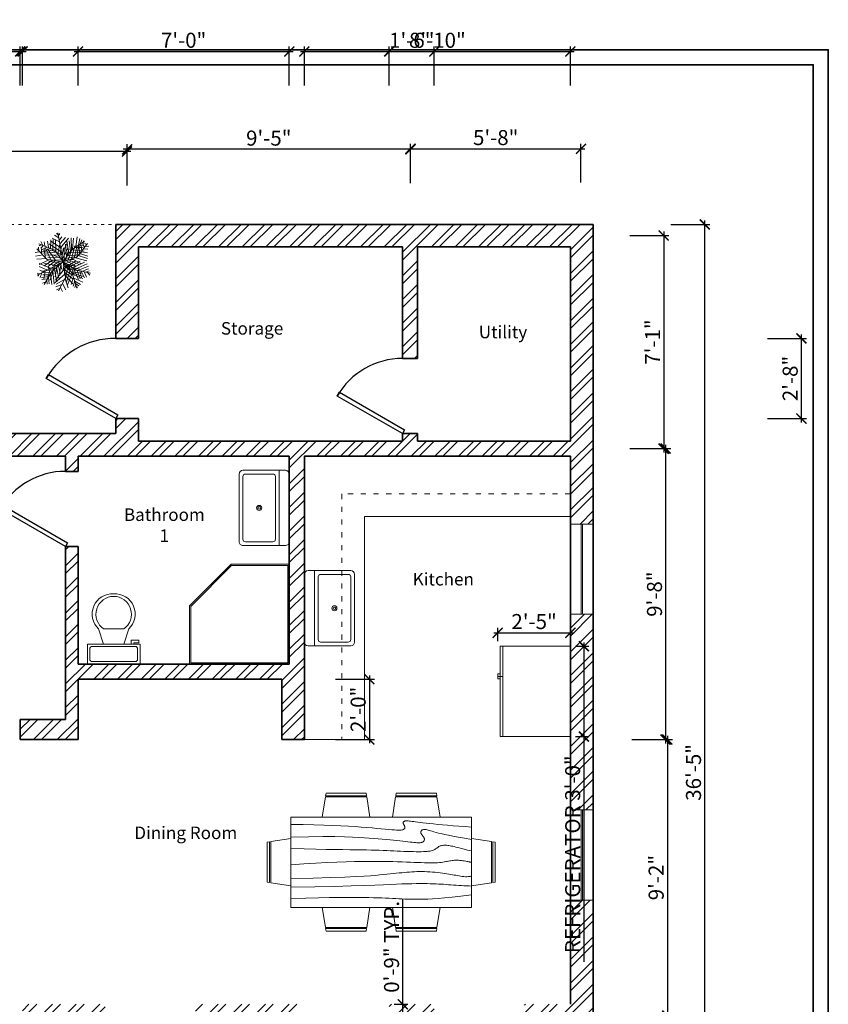
# Model space of a CAD drawing. Units: inches. Extents: x 163 to 947, y 159 to 804.
# Tile 5 of 5: x 625 to 947, y 412 to 804. Entities that reach past the tile are written whole.
import ezdxf

# ---------------------------------------------------------------- set-up
doc = ezdxf.new("R2010")
doc.units = ezdxf.units.IN
doc.linetypes.add('ACAD_ISO03W100', pattern=[30, 12, -18])
for name, color, linetype, lineweight in [('A-ANNO-TTLB', 7, 'Continuous', 35), ('A-AREA-IDEN', 7, 'Continuous', 18), ('A-EQPM', 121, 'Continuous', 18), ('A-FLOR-CASE', 7, 'Continuous', 18), ('A-FLOR-CASE-OVHD', 7, 'ACAD_ISO03W100', 18), ('A-FLOR-FIXT', 121, 'Continuous', 18), ('A-ROOF-OVHD', 7, 'ACAD_ISO03W100', 18), ('Dimensions', 7, 'Continuous', 18), ('Doors', 160, 'Continuous', 25), ('Furniture', 40, 'Continuous', 18), ('Greenary  Plants', 100, 'Continuous', 13), ('Wall Hatch', 214, 'Continuous', 13), ('Walls', 222, 'Continuous', 35), ('Windows', 132, 'Continuous', 18)]:
    doc.layers.add(name, color=color, linetype=linetype, lineweight=lineweight)
doc.styles.get("Standard").update_dxf_attribs({"font": 'arial.ttf'})
doc.dimstyles.new('ISO-25', dxfattribs={"dimtxt": 6, "dimasz": 4, "dimexe": 2, "dimexo": 2, "dimtad": 1, "dimdec": 1, "dimlunit": 3, "dimtxsty": 'Standard', "dimblk": 'ARCHTICK', "dimcen": 0, "dimdle": 1.5, "dimadec": 0, "dimazin": 0, "dimtfac": 1, "dimtdec": 1, "dimtmove": 0, "dimatfit": 3, "dimfxl": 13.5, "dimfxlon": 1, "dimarcsym": 0})

# ---------------------------------------------------------------- blocks, each defined once
blk = doc.blocks.new('_ArchTick')
at = {"color": 0, "linetype": 'ByBlock', "const_width": 0.15}
blk.add_lwpolyline([(-0.5, -0.5), (0.5, 0.5)], dxfattribs=at)
blk = doc.blocks.new('*D2')
at = {"layer": 'Dimensions', "color": 0, "lineweight": -2, "transparency": 16777216}
for p, q in [((780.8, 739.36), (780.8, 754.86)), ((848.8, 739.36), (848.8, 754.86)), ((779.3, 752.86), (850.3, 752.86))]:
    blk.add_line(p, q, dxfattribs=at)
at = {"layer": 'Dimensions', "color": 0, "lineweight": -2, "transparency": 16777216, "xscale": 4, "yscale": 4, "zscale": 4, "rotation": 180}
blk.add_blockref('_ArchTick', (780.8, 752.86), dxfattribs=at)
at = {"layer": 'Dimensions', "color": 0, "lineweight": -2, "transparency": 16777216, "xscale": 4, "yscale": 4, "zscale": 4}
blk.add_blockref('_ArchTick', (848.8, 752.86), dxfattribs=at)
at = {"layer": 'Dimensions', "color": 0, "transparency": 16777216, "insert": (814.8, 756.55), "char_height": 6, "attachment_point": 5}
blk.add_mtext('5\'-8"', dxfattribs=at)
blk = doc.blocks.new('*D3')
at = {"layer": 'Dimensions', "color": 0, "lineweight": -2, "transparency": 16777216}
for p, q in [((667.8, 739.15), (667.8, 754.65)), ((780.8, 739.15), (780.8, 754.65)), ((782.3, 752.65), (666.3, 752.65))]:
    blk.add_line(p, q, dxfattribs=at)
at = {"layer": 'Dimensions', "color": 0, "lineweight": -2, "transparency": 16777216, "xscale": 4, "yscale": 4, "zscale": 4, "rotation": 180}
blk.add_blockref('_ArchTick', (667.8, 752.65), dxfattribs=at)
at = {"layer": 'Dimensions', "color": 0, "lineweight": -2, "transparency": 16777216, "xscale": 4, "yscale": 4, "zscale": 4}
blk.add_blockref('_ArchTick', (780.8, 752.65), dxfattribs=at)
at = {"layer": 'Dimensions', "color": 0, "transparency": 16777216, "insert": (724.3, 756.34), "char_height": 6, "attachment_point": 5}
blk.add_mtext('9\'-5"', dxfattribs=at)
blk = doc.blocks.new('*D4')
at = {"layer": 'Dimensions', "color": 0, "lineweight": -2, "transparency": 16777216}
for p, q in [((542.8, 738.28), (542.8, 753.78)), ((667.8, 738.28), (667.8, 753.78)), ((669.3, 751.78), (541.3, 751.78))]:
    blk.add_line(p, q, dxfattribs=at)
at = {"layer": 'Dimensions', "color": 0, "lineweight": -2, "transparency": 16777216, "xscale": 4, "yscale": 4, "zscale": 4, "rotation": 180}
blk.add_blockref('_ArchTick', (542.8, 751.78), dxfattribs=at)
at = {"layer": 'Dimensions', "color": 0, "lineweight": -2, "transparency": 16777216, "xscale": 4, "yscale": 4, "zscale": 4}
blk.add_blockref('_ArchTick', (667.8, 751.78), dxfattribs=at)
at = {"layer": 'Dimensions', "color": 0, "transparency": 16777216, "insert": (605.3, 755.47), "char_height": 6, "attachment_point": 5}
blk.add_mtext('10\'-5"', dxfattribs=at)
blk = doc.blocks.new('*D8')
at = {"layer": 'Dimensions', "color": 0, "lineweight": -2, "transparency": 16777216}
for p, q in [((881.79, 719.82), (881.79, 631.82)), ((868.29, 718.32), (883.79, 718.32)), ((868.29, 633.32), (883.79, 633.32))]:
    blk.add_line(p, q, dxfattribs=at)
at = {"layer": 'Dimensions', "color": 0, "lineweight": -2, "transparency": 16777216, "xscale": 4, "yscale": 4, "zscale": 4}
for p, rotation in [((881.79, 718.32), 90), ((881.79, 633.32), 270)]:
    blk.add_blockref('_ArchTick', p, dxfattribs=dict(at, rotation=rotation))
at = {"layer": 'Dimensions', "color": 0, "transparency": 16777216, "insert": (878.15, 675.82), "char_height": 6, "attachment_point": 5, "rotation": 90}
blk.add_mtext('7\'-1"', dxfattribs=at)
blk = doc.blocks.new('*D9')
at = {"layer": 'Dimensions', "color": 0, "lineweight": -2, "transparency": 16777216}
for p, q in [((869.08, 633.32), (884.58, 633.32)), ((882.58, 634.82), (882.58, 515.82)), ((869.08, 517.32), (884.58, 517.32))]:
    blk.add_line(p, q, dxfattribs=at)
at = {"layer": 'Dimensions', "color": 0, "lineweight": -2, "transparency": 16777216, "xscale": 4, "yscale": 4, "zscale": 4}
for p, rotation in [((882.58, 633.32), 90), ((882.58, 517.32), 270)]:
    blk.add_blockref('_ArchTick', p, dxfattribs=dict(at, rotation=rotation))
at = {"layer": 'Dimensions', "color": 0, "transparency": 16777216, "insert": (878.9, 575.32), "char_height": 6, "attachment_point": 5, "rotation": 90}
blk.add_mtext('9\'-8"', dxfattribs=at)
blk = doc.blocks.new('*D10')
at = {"layer": 'Dimensions', "color": 0, "lineweight": -2, "transparency": 16777216}
for p, q in [((883.25, 518.82), (883.25, 405.78)), ((869.75, 517.32), (885.25, 517.32)), ((869.75, 407.28), (885.25, 407.28))]:
    blk.add_line(p, q, dxfattribs=at)
at = {"layer": 'Dimensions', "color": 0, "lineweight": -2, "transparency": 16777216, "xscale": 4, "yscale": 4, "zscale": 4}
for p, rotation in [((883.25, 517.32), 90), ((883.25, 407.28), 270)]:
    blk.add_blockref('_ArchTick', p, dxfattribs=dict(at, rotation=rotation))
at = {"layer": 'Dimensions', "color": 0, "transparency": 16777216, "insert": (879.57, 462.3), "char_height": 6, "attachment_point": 5, "rotation": 90}
blk.add_mtext('9\'-2"', dxfattribs=at)
blk = doc.blocks.new('*U25')
for p, q in [((-30, 0), (-30, 4)), ((0, 0), (0, 4))]:
    blk.add_line(p, q)
blk.add_lwpolyline([(0, 0), (-15, -25.98), (-16.52, -25.11), (-1.52, 0.87)], close=True)
blk.add_arc((0, 0), 30, 180, 240)
blk = doc.blocks.new('*U26')
for p, q in [((-32, 0), (-32, 4)), ((0, 0), (0, 4))]:
    blk.add_line(p, q)
blk.add_lwpolyline([(0, 0), (-16, -27.71), (-17.52, -26.84), (-1.52, 0.87)], close=True)
blk.add_arc((0, 0), 32, 180, 240)
blk = doc.blocks.new('Dining Set - 36 x 72 in.')
for p, q in [((-22, 27.5), (-22.1562, 26.50042)), ((-22, 27.5), (-6, 27.5)), ((-5.8437, 26.49966), (-6, 27.5)), ((6, 27.5), (5.8438, 26.50042)), ((6, 27.5), (22, 27.5)), ((22.1563, 26.49966), (22, 27.5)), ((-22.2343, 26.00059), (-23.4847, 17.99762)), ((-22.2304, 26), (-5.7608, 26)), ((-5.8416, 26.5), (-22.1534, 26.5)), ((-4.5152, 17.99762), (-5.7655, 25.99926)), ((5.7657, 26.00059), (4.5153, 17.99762)), ((5.7696, 26), (22.2392, 26)), ((22.1584, 26.5), (5.8466, 26.5)), ((23.4848, 17.99762), (22.2345, 25.99926)), ((36, 18), (-36, 18)), ((-36, 18), (-36, -18)), ((36, -18), (36, 18)), ((-45.5, 8), (-44.5004, 8.15617)), ((-45.5, 8), (-45.5, -8)), ((-44.5, -8.15843), (-44.5, 8.15338)), ((-44.0006, 8.23428), (-35.9976, 9.48474)), ((-44, 8.23041), (-44, -8.23915)), ((44.0006, 8.23428), (35.9976, 9.48474)), ((44, 8.23041), (44, -8.23915)), ((44.5, -8.15843), (44.5, 8.15338)), ((45.5, 8), (44.5005, 8.15617)), ((45.5, 8), (45.5, -8)), ((-44.4997, -8.15631), (-45.5, -8)), ((-35.9976, -9.48476), (-43.9993, -8.2345)), ((35.9976, -9.48476), (43.9993, -8.2345)), ((44.4997, -8.15631), (45.5, -8)), ((-36, -18), (36, -18)), ((-22.2343, -26.0006), (-23.4847, -17.99762)), ((-4.5152, -17.99762), (-5.7655, -25.99928)), ((5.7657, -26.0006), (4.5153, -17.99762)), ((23.4848, -17.99762), (22.2345, -25.99928)), ((-22.2304, -26), (-5.7608, -26)), ((-22, -27.5), (-22.1562, -26.50044)), ((-5.8416, -26.5), (-22.1534, -26.5)), ((-5.8437, -26.49967), (-6, -27.5)), ((5.7696, -26), (22.2392, -26)), ((6, -27.5), (5.8438, -26.50044)), ((22.1584, -26.5), (5.8466, -26.5)), ((22.1563, -26.49967), (22, -27.5)), ((-22, -27.5), (-6, -27.5)), ((6, -27.5), (22, -27.5))]:
    blk.add_line(p, q)
for points in [[(-36, 15), (-31.1772, 14.97754), (-26.8079, 14.91406), (-22.8538, 14.81543), (-19.276, 14.6875), (-16.0362, 14.53613), (-13.0957, 14.36718), (-10.4159, 14.18652), (-7.9583, 14), (-5.6904, 13.81315), (-3.6035, 13.63021), (-1.6954, 13.45508), (0.0365, 13.29166), (1.5945, 13.14388), (2.9811, 13.01562), (4.1988, 12.9108), (5.25, 12.83333), (6.1393, 12.78613), (6.8802, 12.76823), (7.4883, 12.77767), (7.9792, 12.8125), (8.3685, 12.87077), (8.6719, 12.95052), (8.9049, 13.0498), (9.0833, 13.16666), (9.2205, 13.29899), (9.3216, 13.44401), (9.3895, 13.59879), (9.4271, 13.76041), (9.4373, 13.92594), (9.4232, 14.09245), (9.3875, 14.257), (9.3333, 14.41666), (9.2638, 14.56917), (9.1836, 14.71484), (9.0975, 14.85465), (9.0104, 14.98958), (8.9272, 15.1206), (8.8529, 15.2487), (8.7922, 15.37483), (8.75, 15.5), (8.7305, 15.62467), (8.7344, 15.74739), (8.7617, 15.86621), (8.8125, 15.97916), (8.8867, 16.08431), (8.9844, 16.17968), (9.1055, 16.26334), (9.25, 16.33333), (9.4189, 16.38802), (9.6172, 16.42708), (9.8506, 16.45052), (10.125, 16.45833), (10.4463, 16.45052), (10.8203, 16.42708), (11.2529, 16.38802), (11.75, 16.33333), (12.3184, 16.26318), (12.9694, 16.17838), (13.7151, 16.07991), (14.5677, 15.96875), (15.5395, 15.84586), (16.6426, 15.71224), (17.8893, 15.56884), (19.2917, 15.41666), (20.859, 15.25667), (22.5879, 15.08984), (24.4721, 14.91715), (26.5052, 14.73958), (28.6809, 14.5581), (30.9929, 14.3737), (33.4347, 14.18733), (36, 14)], [(-36, 10), (-28.9766, 10.14274), (-23.1725, 10.20442), (-18.4241, 10.19775), (-14.5677, 10.13541), (-11.4399, 10.03011), (-8.877, 9.89453), (-6.7154, 9.74137), (-4.7917, 9.58333), (-2.9698, 9.43082), (-1.2246, 9.28515), (0.4415, 9.14534), (2.026, 9.01041), (3.5266, 8.87939), (4.9408, 8.7513), (6.266, 8.62516), (7.5, 8.5), (8.6411, 8.37549), (9.6914, 8.2539), (10.6538, 8.13818), (11.5312, 8.03125), (12.3267, 7.93603), (13.043, 7.85547), (13.6831, 7.79248), (14.25, 7.75), (14.7471, 7.7303), (15.1797, 7.73307), (15.5537, 7.75732), (15.875, 7.80208), (16.1494, 7.86637), (16.3828, 7.94922), (16.5811, 8.04964), (16.75, 8.16666), (16.8944, 8.29915), (17.0143, 8.44531), (17.1089, 8.60319), (17.1771, 8.77083), (17.218, 8.94629), (17.2305, 9.1276), (17.2137, 9.31282), (17.1667, 9.5), (17.0895, 9.6875), (16.987, 9.875), (16.8649, 10.0625), (16.7292, 10.25), (16.5856, 10.4375), (16.4401, 10.625), (16.2985, 10.8125), (16.1667, 11), (16.05, 11.18733), (15.9518, 11.3737), (15.8752, 11.5581), (15.8229, 11.73958), (15.798, 11.91715), (15.8034, 12.08984), (15.842, 12.25667), (15.9167, 12.41666), (16.0295, 12.56836), (16.1784, 12.70833), (16.3605, 12.83268), (16.5729, 12.9375), (16.8127, 13.01888), (17.0768, 13.07291), (17.3625, 13.0957), (17.6667, 13.08333), (17.9894, 13.03312), (18.3418, 12.94726), (18.7382, 12.82918), (19.1927, 12.68229), (19.7195, 12.51001), (20.3327, 12.31575), (21.0465, 12.10294), (21.875, 11.875), (22.8357, 11.63354), (23.959, 11.37304), (25.2786, 11.08618), (26.8282, 10.76562), (28.6414, 10.40405), (30.752, 9.99414), (33.1936, 9.52856), (36, 9)], [(-36, 5.5), (-30.7157, 5.3348), (-26.069, 5.20963), (-21.9946, 5.11767), (-18.4271, 5.05208), (-15.3009, 5.00602), (-12.5508, 4.97265), (-10.1112, 4.94515), (-7.9167, 4.91666), (-5.909, 4.88167), (-4.0586, 4.83984), (-2.3429, 4.79215), (-0.7396, 4.73958), (0.7739, 4.6831), (2.22, 4.6237), (3.6213, 4.56233), (5, 4.5), (6.373, 4.43782), (7.7344, 4.3776), (9.0723, 4.32129), (10.375, 4.27083), (11.6309, 4.22819), (12.8281, 4.19531), (13.9551, 4.17415), (15, 4.16666), (15.954, 4.17448), (16.819, 4.19791), (17.6001, 4.23698), (18.3021, 4.29166), (18.9299, 4.36198), (19.4883, 4.44791), (19.9823, 4.54948), (20.4167, 4.66666), (20.7969, 4.79899), (21.1302, 4.94401), (21.4245, 5.09879), (21.6875, 5.26041), (21.9271, 5.42594), (22.1511, 5.59245), (22.3672, 5.757), (22.5834, 5.91666), (22.8065, 6.06868), (23.0404, 6.21093), (23.2879, 6.34147), (23.5521, 6.45833), (23.8358, 6.55957), (24.142, 6.64323), (24.4735, 6.70735), (24.8334, 6.75), (25.2235, 6.76969), (25.642, 6.76692), (26.0858, 6.74267), (26.5521, 6.69791), (27.0379, 6.63362), (27.5404, 6.55078), (28.0565, 6.45036), (28.5834, 6.33333), (29.1242, 6.19987), (29.7071, 6.04687), (30.3661, 5.87044), (31.1354, 5.66666), (32.0493, 5.43164), (33.142, 5.16146), (34.4475, 4.85221), (36, 4.5)], [(-36, -1), (-30.7915, -0.6591), (-26.0195, -0.38216), (-21.6519, -0.16284), (-17.6563, 0.00521), (-14.0005, 0.12833), (-10.6523, 0.21289), (-7.5796, 0.26522), (-4.75, 0.29166), (-2.134, 0.29793), (0.2878, 0.28711), (2.5317, 0.26163), (4.6146, 0.22396), (6.5529, 0.17651), (8.3633, 0.12174), (10.0623, 0.06209), (11.6667, 0), (13.1899, -0.06201), (14.6341, -0.1211), (15.9982, -0.17432), (17.2813, -0.21875), (18.4823, -0.25147), (19.6003, -0.26953), (20.6343, -0.27002), (21.5834, -0.25), (22.4481, -0.20768), (23.2357, -0.14584), (23.9549, -0.06836), (24.6146, 0.02083), (25.2235, 0.11784), (25.7904, 0.21875), (26.3241, 0.31966), (26.8334, 0.41666), (27.3265, 0.50618), (27.8099, 0.58593), (28.2894, 0.65397), (28.7709, 0.70833), (29.2601, 0.74707), (29.763, 0.76823), (30.2855, 0.76985), (30.8334, 0.75), (31.4088, 0.70784), (31.9994, 0.64713), (32.589, 0.57275), (33.1615, 0.48958), (33.7008, 0.4025), (34.1908, 0.3164), (34.6153, 0.23616), (34.9584, 0.16666), (35.2099, 0.11165), (35.3848, 0.07031), (35.504, 0.04069), (35.5886, 0.02083), (35.6594, 0.00879), (35.7377, 0.0026), (35.8442, 0.00032), (36, 0)], [(-36, -6.5), (-27.1843, -6.31267), (-20.084, -6.1263), (-14.469, -5.9419), (-10.1094, -5.76042), (-6.7752, -5.58285), (-4.2363, -5.41016), (-2.2629, -5.24333), (-0.625, -5.08334), (0.8708, -4.93099), (2.2715, -4.78646), (3.5872, -4.64974), (4.8281, -4.52084), (6.0046, -4.39974), (7.127, -4.28646), (8.2053, -4.18099), (9.25, -4.08334), (10.2705, -3.99382), (11.2734, -3.91407), (12.2647, -3.84603), (13.25, -3.79167), (14.2354, -3.75293), (15.2266, -3.73177), (16.2295, -3.73015), (17.25, -3.75), (18.2912, -3.79248), (19.3451, -3.85547), (20.4009, -3.93604), (21.4479, -4.03125), (22.4754, -4.13819), (23.4727, -4.25391), (24.4289, -4.37549), (25.3334, -4.5), (26.1785, -4.62492), (26.9694, -4.74935), (27.7145, -4.87281), (28.4219, -4.99479), (29.1, -5.11483), (29.7572, -5.23242), (30.4016, -5.34709), (31.0417, -5.45834), (31.6837, -5.56437), (32.3262, -5.65821), (32.9658, -5.73153), (33.599, -5.77604), (34.2224, -5.78345), (34.8327, -5.74545), (35.4264, -5.65373), (36, -5.5)], [(-36, -10), (-26.4022, -9.81299), (-18.4675, -9.62891), (-11.9839, -9.45069), (-6.7396, -9.28125), (-2.5226, -9.12354), (0.8789, -8.98047), (3.6769, -8.85498), (6.0833, -8.75), (8.2767, -8.66765), (10.3021, -8.60677), (12.1712, -8.56543), (13.8958, -8.54167), (15.4876, -8.53353), (16.9583, -8.53907), (18.3197, -8.55632), (19.5834, -8.58334), (20.7616, -8.61841), (21.8685, -8.66081), (22.9188, -8.71004), (23.9271, -8.76563), (24.9081, -8.82707), (25.8763, -8.89388), (26.8465, -8.96558), (27.8334, -9.04167), (28.8474, -9.12118), (29.8828, -9.20117), (30.93, -9.27824), (31.9792, -9.34896), (33.0205, -9.40991), (34.0443, -9.45768), (35.0407, -9.48885), (36, -9.5)], [(-36, -14.5), (-30.0881, -14.33513), (-25.0332, -14.21224), (-20.7312, -14.12647), (-17.0781, -14.07292), (-13.97, -14.04671), (-11.3027, -14.04297), (-8.9724, -14.05681), (-6.875, -14.08334), (-4.9224, -14.11833), (-3.0905, -14.16016), (-1.3709, -14.20785), (0.2448, -14.26042), (1.7647, -14.3169), (3.1973, -14.3763), (4.5507, -14.43767), (5.8333, -14.5), (7.0554, -14.5621), (8.235, -14.62175), (9.3922, -14.67652), (10.5469, -14.72396), (11.7192, -14.76164), (12.929, -14.78711), (14.1965, -14.79794), (15.5417, -14.79167), (16.9933, -14.76424), (18.6152, -14.70508), (20.4804, -14.60197), (22.6615, -14.44271), (25.2312, -14.21509), (28.2624, -13.9069), (31.8277, -13.50594), (36, -13)]]:
    blk.add_lwpolyline(points)
blk = doc.blocks.new('*U50')
for p, q in [((9.5, -6), (9.5, -2)), ((-10, -8.5), (-8, -8.5)), ((-10, -9.5), (-10, -8.5)), ((-7, -9.5), (-10, -9.5)), ((-8, -8.5), (-8, -8)), ((-7, -8), (-7, -9.5)), ((-4, -8), (-6, -14)), ((4, -8), (6, -14)), ((4, -14), (-4, -14))]:
    blk.add_line(p, q)
blk.add_lwpolyline([(10.5, -8), (10.5, 0), (-10.5, 0), (-10.5, -8)], close=True)
for points in [[(-9.5, -2), (-9.5, -6)], [(8.5, -1), (-8.5, -1)], [(-8.5, -7), (8.5, -7)]]:
    blk.add_lwpolyline(points)
for centre, radius, start, end in [((-8.625, -1.875), 0.8839, 81.8699, 188.1301), ((8.625, -1.875), 0.8839, 351.8699, 98.1301), ((-8.625, -6.125), 0.8839, 171.869898, 278.1301), ((8.625, -6.125), 0.8839, 261.8699, 8.1301), ((-0.4772, -19.9188), 8.0953, 133.01722, 273.38), ((0.0374, -19.8731), 7.127, 124.50543, 269.7), ((-0.0373, -19.8731), 7.127, 270.3, 55.4946), ((0.4773, -19.9188), 8.0953, 266.62, 46.9828)]:
    blk.add_arc(centre, radius, start, end)
blk = doc.blocks.new('Sink-single - 30 in top')
blk.add_line((-15, -3.999996), (15, -3.999996))
for points in [[(-13.5, 0), (13.5, 0)], [(-15, -18.499996), (-15, -1.5)], [(15, -1.5), (15, -18.499996)], [(-13.5, -17.499996), (-13.5, -6.499996)], [(-12.5, -5.499996), (12.5, -5.499996)], [(13.5, -6.499996), (13.5, -17.499996)], [(12.5, -18.499996), (-12.5, -18.499996)], [(13.5, -19.999996), (-13.5, -19.999996)]]:
    blk.add_lwpolyline(points)
for radius in [1, 0.5]:
    blk.add_circle((0, -11.999996), radius)
for centre, radius, start, end in [((-13.5, -1.5), 1.5, 90, 180), ((13.5, -1.5), 1.5, 0, 90), ((-12.5, -6.499996), 1, 90, 180), ((12.5, -6.499996), 1, 0, 90), ((-13.5, -18.499996), 1.5, 180, 270), ((-12.5, -17.499996), 1, 180, 270), ((12.5, -17.499996), 1, 270, 0), ((13.5, -18.499996), 1.5, 270, 0)]:
    blk.add_arc(centre, radius, start, end)
blk = doc.blocks.new('Refrigerator-2 door - 36 in top')
for p, q in [((0, -26.999999), (36, -26.999999)), ((12, -26.999999), (12, -28.999999)), ((11, -27.999999), (11, -28.999999)), ((11, -28.999999), (13, -28.999999)), ((13, -28.999999), (13, -27.999999))]:
    blk.add_line(p, q)
blk.add_lwpolyline([(0, -27.999999), (0, 0), (36, 0), (36, -27.999999)], close=True)
blk = doc.blocks.new('*U54')
for p, q in [((-5.114, 28.097), (-24.676, 40.636)), ((-7.288, 39.707), (-21.778, 46.673)), ((-8.737, 47.138), (-17.069, 52.711)), ((-10.186, 53.64), (-13.084, 55.962)), ((0, 0), (-10.5, 57)), ((-9.099, 51.782), (-6.563, 55.962)), ((-7.65, 43.423), (-2.578, 49.46)), ((-5.839, 35.992), (4.667, 48.067)), ((-5.114, 27.632), (10.463, 46.673)), ((-47.498, 19.737), (-55.83, 18.344)), ((-31.5, 4.5), (-52.5, 25.5)), ((-48.585, 21.131), (-49.309, 29.026)), ((-43.513, 28.561), (-42.427, 15.558)), ((-38.442, 26.239), (-34.819, 7.663)), ((-35.544, 28.097), (-24.314, 3.947)), ((-14.533, 2.09), (-30.834, 25.31)), ((-3.665, 19.273), (-27.574, 35.527)), ((-24.314, 23.917), (-2.941, 13.7)), ((-2.941, 16.486), (8.652, 37.85)), ((-1.129, 6.734), (9.014, 26.704)), ((3.942, 1.625), (11.187, 24.381)), ((10.101, 3.483), (17.708, 26.239)), ((16.259, 5.805), (23.142, 31.348)), ((22.055, 7.198), (27.489, 32.277)), ((27, 9), (48, 36)), ((27.127, 9.056), (31.112, 35.992)), ((31.836, 30.883), (32.561, 16.486)), ((35.096, 32.741), (37.27, 22.524)), ((36.183, 19.737), (48.137, 17.88)), ((38.719, 34.134), (41.979, 28.561)), ((40.53, 25.775), (48.862, 24.846)), ((43.791, 29.954), (51.036, 30.883)), ((44.153, 36.456), (45.239, 32.741)), ((-40.615, 13.7), (-55.105, 10.913)), ((-33.37, 6.269), (-52.207, 5.34)), ((-28.299, 3.483), (-47.86, -5.805)), ((-21.416, 3.018), (-38.079, -8.128)), ((0, 0), (-31.5, 4.5)), ((-15.982, 2.09), (-30.11, -9.521)), ((0, 0), (-22.5, -19.5)), ((-6.563, 1.161), (-21.416, -8.128)), ((-20.691, 13.7), (-1.129, 4.876)), ((0, 0), (27, 9)), ((0, 0), (18, -22.5)), ((6.478, 1.625), (26.04, -8.592)), ((11.187, 3.483), (30.749, -5.805)), ((18.07, 5.805), (35.096, -3.483)), ((24.229, 7.663), (46.688, 1.625)), ((29.662, 12.307), (48.137, 6.269)), ((33.285, 16.486), (48.862, 10.913)), ((-17.431, -15.094), (-42.789, -18.809)), ((-22.5, -19.5), (-37.5, -45)), ((-15.257, -12.772), (-30.11, -12.772)), ((-20.691, -18.345), (-17.793, -44.352)), ((-6.563, -5.805), (-19.967, -9.985)), ((-17.069, -15.094), (-12.721, -40.172)), ((-13.446, -11.378), (-8.737, -32.741)), ((-9.461, -8.592), (-6.201, -23.453)), ((-4.752, -3.483), (-3.665, -14.629)), ((2.493, -3.019), (-1.491, -20.202)), ((1.769, -2.555), (24.229, -9.521)), ((5.029, -6.27), (2.131, -25.775)), ((9.014, -11.378), (3.58, -35.992)), ((14.085, -16.951), (6.478, -40.172)), ((7.565, -9.056), (32.198, -14.629)), ((12.274, -15.094), (36.907, -18.809)), ((-28.299, -29.026), (-42.789, -31.348)), ((-24.314, -21.596), (-42.427, -22.06)), ((-30.834, -34.135), (-42.427, -35.528)), ((-26.849, -26.24), (-40.253, -25.775)), ((-32.646, -36.921), (-31.921, -44.352)), ((-29.023, -30.884), (-27.936, -43.887)), ((-25.038, -23.918), (-22.865, -45.281)), ((18.07, -22.524), (8.289, -45.745)), ((20.244, -30.419), (15.897, -44.816)), ((16.259, -19.738), (36.183, -22.989)), ((18, -22.5), (27, -52.5)), ((18.433, -22.524), (40.53, -29.026)), ((19.157, -25.311), (38.719, -33.206)), ((22.78, -37.85), (19.519, -48.532)), ((21.331, -32.741), (39.081, -40.636)), ((22.78, -38.314), (34.372, -44.816)), ((-34.457, -39.708), (-40.978, -42.494)), ((24.591, -45.745), (23.142, -50.854)), ((24.591, -43.423), (30.749, -47.603)), ((26.764, -49.925), (28.213, -50.854))]:
    blk.add_line(p, q)
blk = doc.blocks.new('*D59')
at = {"layer": 'Dimensions', "color": 0, "lineweight": -2, "transparency": 16777216}
for p, q in [((884.65, 722.73), (900.15, 722.73)), ((898.15, 284.27), (898.15, 724.23)), ((884.65, 285.77), (900.15, 285.77))]:
    blk.add_line(p, q, dxfattribs=at)
at = {"layer": 'Dimensions', "color": 0, "lineweight": -2, "transparency": 16777216, "xscale": 4, "yscale": 4, "zscale": 4}
for p, rotation in [((898.15, 722.73), 90), ((898.15, 285.77), 270)]:
    blk.add_blockref('_ArchTick', p, dxfattribs=dict(at, rotation=rotation))
at = {"layer": 'Dimensions', "color": 0, "transparency": 16777216, "insert": (894.46, 504.25), "char_height": 6, "attachment_point": 5, "rotation": 90}
blk.add_mtext('36\'-5"', dxfattribs=at)
blk = doc.blocks.new('WIN-36IN')
for p, q in [((0, 9.03), (0, 0)), ((35.98, 9.03), (35.98, 0)), ((0, 4.76), (35.98, 4.76)), ((0, 4.26), (35.98, 4.26))]:
    blk.add_line(p, q)
blk = doc.blocks.new('*D64')
at = {"layer": 'Dimensions', "color": 0, "lineweight": -2, "transparency": 16777216}
for p, q in [((736.35, 400.77), (736.35, 395.37)), ((772.33, 400.77), (772.33, 395.37)), ((734.85, 397.37), (772.33, 397.37)), ((772.33, 397.37), (853.51, 397.37))]:
    blk.add_line(p, q, dxfattribs=at)
at = {"layer": 'Dimensions', "color": 0, "lineweight": -2, "transparency": 16777216, "xscale": 4, "yscale": 4, "zscale": 4, "rotation": 180}
blk.add_blockref('_ArchTick', (736.35, 397.37), dxfattribs=at)
at = {"layer": 'Dimensions', "color": 0, "lineweight": -2, "transparency": 16777216, "xscale": 4, "yscale": 4, "zscale": 4}
blk.add_blockref('_ArchTick', (772.33, 397.37), dxfattribs=at)
at = {"layer": 'Dimensions', "color": 0, "transparency": 16777216, "insert": (814.92, 401.1), "char_height": 6, "attachment_point": 5}
blk.add_mtext('WINDOW 3\'-0" TYP.', dxfattribs=at)
blk = doc.blocks.new('*D65')
at = {"layer": 'Dimensions', "color": 0, "lineweight": -2, "transparency": 16777216}
for p, q in [((777.73, 411.79), (777.73, 453.62)), ((774.33, 411.79), (779.73, 411.79)), ((777.73, 401.27), (777.73, 411.79)), ((774.33, 402.77), (779.73, 402.77))]:
    blk.add_line(p, q, dxfattribs=at)
at = {"layer": 'Dimensions', "color": 0, "lineweight": -2, "transparency": 16777216, "xscale": 4, "yscale": 4, "zscale": 4}
for p, rotation in [((777.73, 411.79), 90), ((777.73, 402.77), 270)]:
    blk.add_blockref('_ArchTick', p, dxfattribs=dict(at, rotation=rotation))
at = {"layer": 'Dimensions', "color": 0, "transparency": 16777216, "insert": (774.04, 434.7), "char_height": 6, "attachment_point": 5, "rotation": 90}
blk.add_mtext('0\'-9" TYP.', dxfattribs=at)
blk = doc.blocks.new('*D88')
at = {"layer": 'Dimensions', "color": 0, "lineweight": -2, "transparency": 16777216}
for p, q in [((846.6, 554.52), (852, 554.52)), ((850, 556.02), (850, 518.52)), ((846.6, 518.52), (852, 518.52)), ((850, 518.52), (850, 428.7))]:
    blk.add_line(p, q, dxfattribs=at)
at = {"layer": 'Dimensions', "color": 0, "lineweight": -2, "transparency": 16777216, "xscale": 4, "yscale": 4, "zscale": 4}
for p, rotation in [((850, 554.52), 90), ((850, 518.52), 270)]:
    blk.add_blockref('_ArchTick', p, dxfattribs=dict(at, rotation=rotation))
at = {"layer": 'Dimensions', "color": 0, "transparency": 16777216, "insert": (846.27, 471.61), "char_height": 6, "attachment_point": 5, "rotation": 90}
blk.add_mtext('REFRIGERATOR 3\'-0"', dxfattribs=at)
blk = doc.blocks.new('*D89')
at = {"layer": 'Dimensions', "color": 0, "lineweight": -2, "transparency": 16777216}
for p, q in [((815.6, 556.52), (815.6, 561.92)), ((844.6, 556.52), (844.6, 561.92)), ((814.1, 559.92), (846.1, 559.92))]:
    blk.add_line(p, q, dxfattribs=at)
at = {"layer": 'Dimensions', "color": 0, "lineweight": -2, "transparency": 16777216, "xscale": 4, "yscale": 4, "zscale": 4, "rotation": 180}
blk.add_blockref('_ArchTick', (815.6, 559.92), dxfattribs=at)
at = {"layer": 'Dimensions', "color": 0, "lineweight": -2, "transparency": 16777216, "xscale": 4, "yscale": 4, "zscale": 4}
blk.add_blockref('_ArchTick', (844.6, 559.92), dxfattribs=at)
at = {"layer": 'Dimensions', "color": 0, "transparency": 16777216, "insert": (830.1, 563.6), "char_height": 6, "attachment_point": 5}
blk.add_mtext('2\'-5"', dxfattribs=at)
blk = doc.blocks.new('*D93')
at = {"layer": 'Dimensions', "color": 0, "lineweight": -2, "transparency": 16777216}
for p, q in [((648.23, 778.15), (648.23, 793.65)), ((732.47, 778.15), (732.47, 793.65)), ((646.73, 791.65), (733.97, 791.65))]:
    blk.add_line(p, q, dxfattribs=at)
at = {"layer": 'Dimensions', "color": 0, "lineweight": -2, "transparency": 16777216, "xscale": 4, "yscale": 4, "zscale": 4, "rotation": 180}
blk.add_blockref('_ArchTick', (648.23, 791.65), dxfattribs=at)
at = {"layer": 'Dimensions', "color": 0, "lineweight": -2, "transparency": 16777216, "xscale": 4, "yscale": 4, "zscale": 4}
blk.add_blockref('_ArchTick', (732.47, 791.65), dxfattribs=at)
at = {"layer": 'Dimensions', "color": 0, "transparency": 16777216, "insert": (690.35, 795.34), "char_height": 6, "attachment_point": 5}
blk.add_mtext('7\'-0"', dxfattribs=at)
blk = doc.blocks.new('*D94')
at = {"layer": 'Dimensions', "color": 0, "lineweight": -2, "transparency": 16777216}
for p, q in [((738.49, 778.15), (738.49, 793.65)), ((844.6, 778.15), (844.6, 793.65)), ((736.99, 791.65), (846.1, 791.65))]:
    blk.add_line(p, q, dxfattribs=at)
at = {"layer": 'Dimensions', "color": 0, "lineweight": -2, "transparency": 16777216, "xscale": 4, "yscale": 4, "zscale": 4, "rotation": 180}
blk.add_blockref('_ArchTick', (738.49, 791.65), dxfattribs=at)
at = {"layer": 'Dimensions', "color": 0, "lineweight": -2, "transparency": 16777216, "xscale": 4, "yscale": 4, "zscale": 4}
blk.add_blockref('_ArchTick', (844.6, 791.65), dxfattribs=at)
at = {"layer": 'Dimensions', "color": 0, "transparency": 16777216, "insert": (791.54, 795.34), "char_height": 6, "attachment_point": 5}
blk.add_mtext('8\'-10"', dxfattribs=at)
blk = doc.blocks.new('*D96')
at = {"layer": 'Dimensions', "color": 0, "lineweight": -2, "transparency": 16777216}
for p, q in [((923.2, 677.29), (938.7, 677.29)), ((936.7, 643.79), (936.7, 678.79)), ((923.2, 645.29), (938.7, 645.29))]:
    blk.add_line(p, q, dxfattribs=at)
at = {"layer": 'Dimensions', "color": 0, "lineweight": -2, "transparency": 16777216, "xscale": 4, "yscale": 4, "zscale": 4}
for p, rotation in [((936.7, 677.29), 90), ((936.7, 645.29), 270)]:
    blk.add_blockref('_ArchTick', p, dxfattribs=dict(at, rotation=rotation))
at = {"layer": 'Dimensions', "color": 0, "transparency": 16777216, "insert": (933.01, 661.29), "char_height": 6, "attachment_point": 5, "rotation": 90}
blk.add_mtext('2\'-8"', dxfattribs=at)
blk = doc.blocks.new('*D98')
at = {"layer": 'Dimensions', "color": 0, "lineweight": -2, "transparency": 16777216}
for p, q in [((772.33, 778.15), (772.33, 793.65)), ((790.32, 778.15), (790.32, 793.65)), ((770.83, 791.65), (791.82, 791.65))]:
    blk.add_line(p, q, dxfattribs=at)
at = {"layer": 'Dimensions', "color": 0, "lineweight": -2, "transparency": 16777216, "xscale": 4, "yscale": 4, "zscale": 4, "rotation": 180}
blk.add_blockref('_ArchTick', (772.33, 791.65), dxfattribs=at)
at = {"layer": 'Dimensions', "color": 0, "lineweight": -2, "transparency": 16777216, "xscale": 4, "yscale": 4, "zscale": 4}
blk.add_blockref('_ArchTick', (790.32, 791.65), dxfattribs=at)
at = {"layer": 'Dimensions', "color": 0, "transparency": 16777216, "insert": (781.33, 795.34), "char_height": 6, "attachment_point": 5}
blk.add_mtext('1\'-6"', dxfattribs=at)
blk = doc.blocks.new('*D99')
at = {"layer": 'Dimensions', "color": 0, "lineweight": -2, "transparency": 16777216}
for p, q in [((528.33, 778.15), (528.33, 793.65)), ((626.1, 778.15), (626.1, 793.65)), ((526.83, 791.65), (627.6, 791.65))]:
    blk.add_line(p, q, dxfattribs=at)
at = {"layer": 'Dimensions', "color": 0, "lineweight": -2, "transparency": 16777216, "xscale": 4, "yscale": 4, "zscale": 4, "rotation": 180}
blk.add_blockref('_ArchTick', (528.33, 791.65), dxfattribs=at)
at = {"layer": 'Dimensions', "color": 0, "lineweight": -2, "transparency": 16777216, "xscale": 4, "yscale": 4, "zscale": 4}
blk.add_blockref('_ArchTick', (626.1, 791.65), dxfattribs=at)
at = {"layer": 'Dimensions', "color": 0, "transparency": 16777216, "insert": (577.22, 795.34), "char_height": 6, "attachment_point": 5}
blk.add_mtext('8\'-2"', dxfattribs=at)
blk = doc.blocks.new('*D100')
at = {"layer": 'Dimensions', "color": 0, "lineweight": -2, "transparency": 16777216}
for p, q in [((546.44, 778.15), (546.44, 793.65)), ((625.17, 778.15), (625.17, 793.65)), ((544.94, 791.65), (626.67, 791.65))]:
    blk.add_line(p, q, dxfattribs=at)
at = {"layer": 'Dimensions', "color": 0, "lineweight": -2, "transparency": 16777216, "xscale": 4, "yscale": 4, "zscale": 4, "rotation": 180}
blk.add_blockref('_ArchTick', (546.44, 791.65), dxfattribs=at)
at = {"layer": 'Dimensions', "color": 0, "lineweight": -2, "transparency": 16777216, "xscale": 4, "yscale": 4, "zscale": 4}
blk.add_blockref('_ArchTick', (625.17, 791.65), dxfattribs=at)
at = {"layer": 'Dimensions', "color": 0, "transparency": 16777216, "insert": (585.81, 795.38), "char_height": 6, "attachment_point": 5}
blk.add_mtext('6\'-6 1/2"', dxfattribs=at)
blk = doc.blocks.new('*D101')
at = {"layer": 'Dimensions', "color": 0, "lineweight": -2, "transparency": 16777216}
for p, q in [((764.42, 542.91), (764.42, 515.84)), ((750.92, 541.41), (766.42, 541.41)), ((750.92, 517.34), (766.42, 517.34))]:
    blk.add_line(p, q, dxfattribs=at)
at = {"layer": 'Dimensions', "color": 0, "lineweight": -2, "transparency": 16777216, "xscale": 4, "yscale": 4, "zscale": 4}
for p, rotation in [((764.42, 541.41), 90), ((764.42, 517.34), 270)]:
    blk.add_blockref('_ArchTick', p, dxfattribs=dict(at, rotation=rotation))
at = {"layer": 'Dimensions', "color": 0, "transparency": 16777216, "insert": (760.73, 529.38), "char_height": 6, "attachment_point": 5, "rotation": 90}
blk.add_mtext('2\'-0"', dxfattribs=at)

msp = doc.modelspace()

# ---------------------------------------------------------------- hatches: boundary and pattern name
at = {"layer": 'Wall Hatch'}
h = msp.add_hatch(dxfattribs=at)
h.set_pattern_fill('ANSI32', color=256, scale=0.7)
h.paths.add_polyline_path([(271.66, 713.71), (308.91, 713.71), (308.91, 722.73), (262.64, 722.73), (262.64, 565.31), (271.66, 565.31), (271.66, 583.27), (310.31, 583.27), (310.31, 587.28), (271.66, 587.28)])
h.paths.add_polyline_path([(357.32, 713.71), (400.68, 713.71), (400.68, 722.73), (344.89, 722.73), (344.89, 713.71), (352.3, 713.71), (352.3, 587.28), (340.31, 587.28), (340.31, 583.27), (387.9, 583.27), (387.9, 580.28), (391.92, 580.28), (391.92, 583.27), (411.3, 583.27), (411.3, 587.28), (357.32, 587.28)])
h.paths.add_polyline_path([(454.65, 722.73), (436.66, 722.73), (436.66, 713.71), (444.3, 713.71), (444.3, 587.28), (441.3, 587.28), (441.3, 583.27), (452.32, 583.27), (452.32, 587.28), (449.32, 587.28), (449.32, 713.71), (454.65, 713.71)])
h.paths.add_polyline_path([(546.44, 722.73), (490.63, 722.73), (490.63, 713.71), (537.42, 713.71), (537.42, 587.28), (482.32, 587.28), (482.32, 583.27), (546.44, 583.27), (546.44, 630.27), (552.44, 630.27), (552.44, 639.3), (546.44, 639.3)])
h.paths.add_polyline_path([(271.66, 529.33), (262.64, 529.33), (262.64, 402.77), (290.54, 402.77), (290.54, 411.79), (271.66, 411.79)])
h.paths.add_polyline_path([(344.49, 408.77), (344.51, 411.79), (326.52, 411.79), (326.52, 402.77), (344.49, 402.77)])
h.paths.add_polyline_path([(528.33, 411.79), (510.34, 411.79), (510.34, 521.35), (546.44, 521.35), (546.44, 525.36), (460.92, 525.36), (460.9, 525.35), (460.9, 521.35), (501.32, 521.35), (501.32, 411.79), (390.5, 411.79), (390.5, 521.35), (430.9, 521.35), (430.9, 525.36), (390.5, 525.36), (390.5, 541.96), (386.49, 541.96), (386.49, 411.79), (380.49, 411.79), (380.49, 402.77), (439.11, 402.77), (439.11, 392.26), (448.14, 392.26), (448.14, 402.77), (528.33, 402.77)])
h.paths.add_polyline_path([(448.14, 356.28), (439.11, 356.28), (439.11, 338.29), (448.14, 338.29)])
h.paths.add_polyline_path([(542.45, 294.79), (448.14, 294.79), (448.14, 302.31), (439.11, 302.31), (439.11, 285.77), (542.45, 285.77)])
h.paths.add_polyline_path([(596.42, 294.79), (578.43, 294.79), (578.43, 285.77), (596.42, 285.77)])
h.paths.add_polyline_path([(653.12, 402.77), (659.11, 402.77), (659.11, 408.77), (659.11, 411.79), (626.1, 411.79), (626.1, 402.77), (644.09, 402.77), (644.09, 294.79), (632.4, 294.79), (632.4, 285.77), (653.12, 285.77)])
h.paths.add_polyline_path([(738.49, 630.27), (844.6, 630.27), (844.6, 603.27), (853.62, 603.27), (853.62, 722.73), (663.29, 722.73), (663.29, 677.29), (672.32, 677.29), (672.32, 713.71), (777.6, 713.71), (777.6, 669.29), (783.62, 669.29), (783.62, 713.71), (844.6, 713.71), (844.6, 636.29), (783.62, 636.29), (783.62, 639.29), (777.6, 639.29), (777.6, 636.29), (672.32, 636.29), (672.32, 645.29), (663.29, 645.29), (663.29, 639.3), (582.43, 639.3), (582.43, 630.27), (643.22, 630.27), (643.22, 624.27), (648.23, 624.27), (648.23, 630.27), (732.47, 630.27), (732.47, 547.43), (648.23, 547.43), (648.23, 594.27), (643.22, 594.27), (643.22, 525.36), (625.17, 525.36), (625.17, 517.34), (648.23, 517.34), (648.23, 541.41), (729.47, 541.41), (729.47, 517.34), (738.49, 517.34)])
h.paths.add_polyline_path([(853.62, 567.29), (844.6, 567.29), (844.6, 489.33), (853.62, 489.33)])
h.paths.add_polyline_path([(853.62, 453.35), (844.6, 453.35), (844.6, 411.79), (826.3, 411.79), (826.3, 402.77), (853.62, 402.77)])
h.paths.add_polyline_path([(790.32, 411.79), (772.33, 411.79), (772.33, 402.77), (790.32, 402.77)])
h.paths.add_polyline_path([(736.35, 411.79), (695.11, 411.79), (695.11, 402.77), (736.35, 402.77)])

# ---------------------------------------------------------------- linework, layer by layer
at = {"layer": 'A-ANNO-TTLB'}
for points in [[(163.29, 792.35), (947.45, 792.35), (947.45, 158.54), (163.29, 158.54)], [(169.29, 786.35), (941.45, 786.35), (941.45, 164.54), (169.29, 164.54)]]:
    msp.add_lwpolyline(points, close=True, dxfattribs=at)
at = {"layer": 'A-FLOR-CASE'}
msp.add_line((762.49, 517.34), (738.49, 517.34), dxfattribs=at)
msp.add_lwpolyline([(844.6, 606.27), (762.49, 606.27), (762.49, 517.34)], dxfattribs=at)
at = {"layer": 'A-FLOR-CASE-OVHD', "ltscale": 0.17}
msp.add_lwpolyline([(844.6, 615.27), (753.49, 615.27), (753.49, 517.34)], dxfattribs=at)
at = {"layer": 'A-FLOR-FIXT'}
for points in [[(692.69, 570.64), (692.69, 547.43), (732.47, 547.43), (732.47, 587.21), (709.26, 587.21)], [(693.19, 570.43), (693.19, 547.93), (731.97, 547.93), (731.97, 586.71), (709.47, 586.71)]]:
    msp.add_lwpolyline(points, close=True, dxfattribs=at)
at = {"layer": 'A-ROOF-OVHD', "ltscale": 0.1}
msp.add_line((546.44, 722.73), (663.29, 722.73), dxfattribs=at)
at = {"layer": 'Walls'}
for p, q in [((853.62, 722.73), (663.29, 722.73)), ((663.29, 722.73), (663.29, 677.29)), ((853.62, 402.77), (853.62, 722.73)), ((672.32, 713.71), (672.32, 677.29)), ((777.6, 713.71), (672.32, 713.71)), ((777.6, 669.29), (777.6, 713.71)), ((844.6, 713.71), (783.62, 713.71)), ((783.62, 669.29), (783.62, 713.71)), ((844.6, 636.29), (844.6, 713.71)), ((663.29, 677.29), (672.32, 677.29)), ((777.6, 669.29), (783.62, 669.29)), ((663.29, 645.29), (672.32, 645.29)), ((663.29, 645.29), (663.29, 639.3)), ((672.32, 645.29), (672.32, 636.29)), ((663.29, 639.3), (582.43, 639.3)), ((777.6, 636.29), (672.32, 636.29)), ((777.6, 636.29), (777.6, 639.29)), ((777.6, 639.29), (783.62, 639.29)), ((783.62, 636.29), (783.62, 639.29)), ((844.6, 636.29), (783.62, 636.29)), ((643.22, 630.27), (582.43, 630.27)), ((643.22, 624.27), (643.22, 630.27)), ((648.23, 624.27), (648.23, 630.27)), ((732.47, 630.27), (648.23, 630.27)), ((732.47, 547.43), (732.47, 630.27)), ((844.6, 411.79), (844.6, 630.27)), ((643.22, 624.27), (648.23, 624.27)), ((643.22, 525.36), (643.22, 594.27)), ((643.22, 594.27), (648.23, 594.27)), ((648.23, 547.43), (648.23, 594.27)), ((732.47, 547.43), (648.23, 547.43)), ((648.23, 517.34), (648.23, 541.41)), ((729.47, 541.41), (648.23, 541.41)), ((729.47, 517.34), (729.47, 541.41)), ((625.17, 517.34), (625.17, 525.36)), ((643.22, 525.36), (625.17, 525.36)), ((648.23, 517.34), (625.17, 517.34)), ((738.49, 517.34), (729.47, 517.34))]:
    msp.add_line(p, q, dxfattribs=at)
msp.add_lwpolyline([(844.6, 630.27), (738.49, 630.27), (738.49, 517.34)], dxfattribs=at)

# ---------------------------------------------------------------- block references
at = {"layer": 'A-EQPM', "rotation": 270}
msp.add_blockref('Refrigerator-2 door - 36 in top', (844.6, 554.52), dxfattribs=at)
at = {"layer": 'A-FLOR-FIXT'}
for name, p, rotation in [('Sink-single - 30 in top', (732.47, 609.69), 270), ('Sink-single - 30 in top', (738.49, 569.68), 90), ('*U50', (662.45, 547.43), 180)]:
    msp.add_blockref(name, p, dxfattribs=dict(at, rotation=rotation))
at = {"layer": 'Doors', "rotation": 270}
for name, p in [('*U26', (663.29, 645.29)), ('*U25', (777.6, 639.29)), ('*U25', (643.22, 594.27))]:
    msp.add_blockref(name, p, dxfattribs=at)
at = {"layer": 'Furniture'}
msp.add_blockref('Dining Set - 36 x 72 in.', (769.13, 468.45), dxfattribs=at)
at = {"layer": 'Greenary  Plants', "xscale": 0.2010375495604706, "yscale": 0.2010375495604706, "zscale": 0.2010375495604706, "rotation": 106.8221293867638}
msp.add_blockref('*U54', (642.32, 707.83), dxfattribs=at)
at = {"layer": 'Greenary  Plants', "xscale": 0.2010375495604706, "yscale": 0.2010375495604706, "zscale": 0.2010375495604706}
msp.add_blockref('*U54', (642.32, 707.83), dxfattribs=at)
at = {"layer": 'Windows'}
for p, rotation in [((853.62, 567.29), 89.99999999999955), ((853.62, 453.35), 89.9999999999994)]:
    msp.add_blockref('WIN-36IN', p, dxfattribs=dict(at, rotation=rotation))

# ---------------------------------------------------------------- texts
at = {"layer": 'A-AREA-IDEN', "char_height": 5, "attachment_point": 1}
for s, width, insert in [('\\pxqc;{\\fTimes New Roman|b0|i0|c0|p18;Storage}', 36.0874, (699.6, 683.77)), ('\\pxqc;{\\fTimes New Roman|b0|i0|c0|p18;Utility}', 36.0874, (799.67, 682.31)), ('\\pxqc;{\\fTimes New Roman|b0|i0|c0|p18;Bathroom 1}', 36.0874, (664.62, 609.49)), ('\\pxqc;{\\fTimes New Roman|b0|i0|c0|p18;Kitchen}', 36.0874, (775.87, 583.77)), ('\\pxqc;{\\fTimes New Roman|b0|i0|c0|p18;Dining Room}', 43.4172, (669.49, 482.66))]:
    msp.add_mtext_dynamic_manual_height_columns(s, width=width, gutter_width=12.5, heights=[0], dxfattribs=dict(at, insert=insert))

# ---------------------------------------------------------------- dimensions: what is measured, and where the dimension line sits
at = {"layer": 'Dimensions'}
for base, p1, p2, override, picture, middle in [((625.17, 791.65), (546.44, 525.36), (625.17, 525.36), {"dimdec": 1, "dimlfac": 1, "dimrnd": 0, "dimzin": 1, "dimdsep": 46, "dimlunit": 4, "dimfrac": 2}, '*D100', (585.81, 795.38)), ((626.1, 791.65), (528.33, 411.79), (626.1, 411.79), {"dimdec": 1, "dimlfac": 1, "dimrnd": 0, "dimzin": 1, "dimdsep": 46, "dimlunit": 4, "dimfrac": 2}, '*D99', (577.22, 795.34)), ((732.47, 791.65), (648.23, 547.43), (732.47, 547.43), {"dimdec": 1, "dimlfac": 1, "dimrnd": 0, "dimzin": 1, "dimdsep": 46, "dimlunit": 4, "dimfrac": 2}, '*D93', (690.35, 795.34)), ((844.6, 791.65), (738.49, 517.34), (844.6, 518.52), {"dimdec": 1, "dimlfac": 1, "dimrnd": 0, "dimzin": 1, "dimdsep": 46, "dimlunit": 4, "dimfrac": 2}, '*D94', (791.54, 795.34)), ((790.32, 791.65), (772.33, 411.79), (790.32, 411.79), {"dimdec": 1, "dimlfac": 1, "dimrnd": 0, "dimzin": 1, "dimdsep": 46, "dimlunit": 4, "dimfrac": 2}, '*D98', (781.33, 795.34)), ((542.8, 751.78), (667.8, 724.34), (542.8, 724.34), {"dimclrd": 0, "dimclre": 0, "dimclrt": 0}, '*D4', (605.3, 755.47)), ((667.8, 752.65), (780.8, 724.34), (667.8, 724.34), {"dimclrd": 0, "dimclre": 0, "dimclrt": 0}, '*D3', (724.3, 756.34)), ((848.8, 752.86), (780.8, 724.34), (848.8, 724.34), {"dimclrd": 0, "dimclre": 0, "dimclrt": 0}, '*D2', (814.8, 756.55)), ((844.6, 559.92), (815.6, 554.52), (844.6, 554.52), {"dimdec": 1, "dimlfac": 1, "dimrnd": 0, "dimzin": 1, "dimdsep": 46, "dimlunit": 4, "dimfrac": 2}, '*D89', (830.1, 563.6))]:
    dim = msp.add_linear_dim(base=base, p1=p1, p2=p2, dimstyle='ISO-25', override=override, dxfattribs=at)
    dim.commit()
    dim.dimension.update_dxf_attribs({"geometry": picture, "text_midpoint": middle})
for base, p1, p2, angle, override, picture, middle in [((898.15, 722.73), (853.62, 285.77), (853.62, 722.73), 90, {"dimclrd": 0, "dimclre": 0, "dimclrt": 0}, '*D59', (894.46, 504.25)), ((881.79, 633.32), (858.02, 718.32), (858.02, 633.32), 90, {"dimclrd": 0, "dimclre": 0, "dimclrt": 0}, '*D8', (878.15, 675.82)), ((936.7, 677.29), (663.29, 645.29), (663.29, 677.29), 90, {"dimdec": 1, "dimlfac": 1, "dimrnd": 0, "dimzin": 1, "dimdsep": 46, "dimlunit": 4, "dimfrac": 2}, '*D96', (933.01, 661.29)), ((882.58, 517.32), (858.02, 633.32), (858.02, 517.32), 90, {"dimclrd": 0, "dimclre": 0, "dimclrt": 0}, '*D9', (878.9, 575.32)), ((764.42, 517.34), (729.47, 541.41), (729.47, 517.34), 270, {"dimdec": 1, "dimlfac": 1, "dimrnd": 0, "dimzin": 1, "dimdsep": 46, "dimlunit": 4, "dimfrac": 2}, '*D101', (760.73, 529.38)), ((883.25, 407.28), (858.02, 517.32), (858.02, 407.28), 90, {"dimclrd": 0, "dimclre": 0, "dimclrt": 0}, '*D10', (879.57, 462.3))]:
    dim = msp.add_linear_dim(base=base, p1=p1, p2=p2, angle=angle, dimstyle='ISO-25', override=override, dxfattribs=at)
    dim.commit()
    dim.dimension.update_dxf_attribs({"geometry": picture, "text_midpoint": middle})
for base, p1, p2, angle, text, picture, middle in [((850, 518.52), (844.6, 554.52), (844.6, 518.52), 270, 'REFRIGERATOR <>', '*D88', (846.27, 471.61)), ((777.73, 411.79), (772.33, 402.77), (772.33, 411.79), 90, '<> TYP.', '*D65', (774.04, 434.7))]:
    dim = msp.add_linear_dim(base=base, p1=p1, p2=p2, angle=angle, text=text, dimstyle='ISO-25', override={"dimdec": 1, "dimlfac": 1, "dimrnd": 0, "dimzin": 1, "dimdsep": 46, "dimlunit": 4, "dimfrac": 2}, dxfattribs=at)
    dim.commit()
    dim.dimension.update_dxf_attribs({"geometry": picture, "text_midpoint": middle})
dim = msp.add_linear_dim(base=(772.33, 397.37), p1=(736.35, 402.77), p2=(772.33, 402.77), text='WINDOW <> TYP.', dimstyle='ISO-25', override={"dimdec": 1, "dimlfac": 1, "dimrnd": 0, "dimzin": 1, "dimdsep": 46, "dimlunit": 4, "dimfrac": 2}, dxfattribs=at)
dim.commit()
dim.dimension.update_dxf_attribs({"geometry": '*D64', "text_midpoint": (814.92, 401.1)})

doc.saveas('drawing.dxf')
